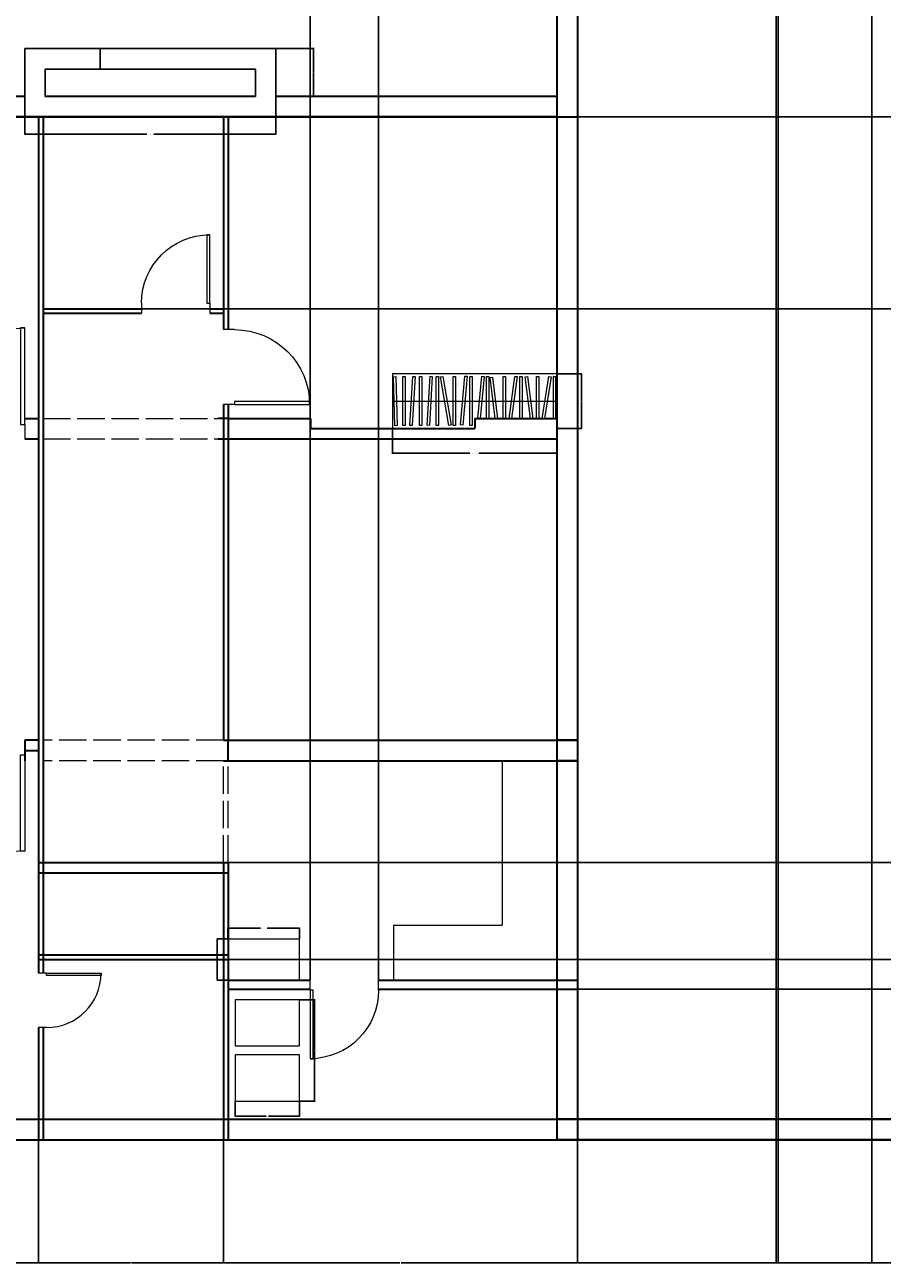
# Model space of a CAD drawing. Units: inches. Extents: x 531915 to 533151, y 849859 to 851471.
# Tile 3 of 7: x 532210 to 532585, y 850315 to 850858. Entities that reach past the tile are written whole.
import ezdxf

# ---------------------------------------------------------------- set-up
doc = ezdxf.new("R2010")
doc.units = ezdxf.units.IN
doc.linetypes.add('ACAD_ISO02W100', pattern=[15, 12, -3])
for name, color, linetype, lineweight in [('A-ANNO-DIMS', 2, 'Continuous', 18), ('A-DOOR', 3, 'Continuous', 18), ('A-FLOR-CASE', 9, 'Continuous', 18), ('A-FLOR-FIXT', 8, 'Continuous', 18), ('A-FLOR-SLAB', 7, 'Continuous', 25), ('A-FURN', 8, 'Continuous', 13), ('A-WALL', 7, 'Continuous', 35), ('A-WALL-OVHD', 7, 'ACAD_ISO02W100', 18)]:
    doc.layers.add(name, color=color, linetype=linetype, lineweight=lineweight)
doc.styles.get("Standard").update_dxf_attribs({"font": 'arial.ttf'})
doc.dimstyles.get("Standard").update_dxf_attribs({"dimtxt": 0.18, "dimasz": 0.18, "dimexe": 0.18, "dimexo": 0.0625, "dimgap": 0.09, "dimtad": 0, "dimtih": 1, "dimtoh": 1, "dimdec": 4, "dimzin": 0, "dimdsep": 46, "dimtxsty": 'Standard', "dimcen": 0.09, "dimadec": 0, "dimazin": 0, "dimtfac": 1, "dimtdec": 4, "dimtofl": 0, "dimtmove": 0, "dimatfit": 3, "dimfxl": 1, "dimtolj": 1, "dimtzin": 0, "dimarcsym": 0})

# ---------------------------------------------------------------- blocks, each defined once
blk = doc.blocks.new('*U2')
for p, q in [((0, 0), (0, -6)), ((40, 0), (40, -6))]:
    blk.add_line(p, q)
blk.add_lwpolyline([(0, 0), (0, 40), (1.75, 40), (1.75, 0)], close=True)
blk.add_arc((0, 0), 40, 0, 90)
blk = doc.blocks.new('WARDROBE-72-RECESSED')
blk.add_line((0, 12), (72, 12))
for points in [[(72, 0), (72, 24), (0, 24), (0, 0), (36.16, 0)], [(37.42, 4.5), (39.13, 22.96), (40.14, 22.87), (38.44, 4.5)], [(41.19, 4.5), (41.19, 22.85), (42.2, 22.85), (42.2, 4.5)], [(45.01, 4.5), (42.84, 22.45), (43.84, 22.58), (46.03, 4.5)], [(48.51, 4.5), (48.51, 22.85), (49.52, 22.85), (49.52, 4.5)], [(51.17, 4.5), (53.59, 22.89), (54.59, 22.76), (52.19, 4.5)], [(55.83, 4.5), (55.83, 22.85), (56.84, 22.85), (56.84, 4.5)], [(60.46, 4.5), (58.13, 22.7), (59.13, 22.83), (61.48, 4.5)], [(63.15, 4.5), (63.15, 22.85), (64.16, 22.85), (64.16, 4.5)], [(65.55, 4.5), (68.56, 22.79), (69.55, 22.63), (66.57, 4.5)], [(70.47, 4.5), (70.47, 22.85), (71.48, 22.85), (71.48, 4.5)]]:
    blk.add_lwpolyline(points)
for points in [[(0.42, 22.75), (1.43, 22.78), (2.11, 1.3), (1.1, 1.27)], [(4.59, 22.85), (5.6, 22.85), (5.6, 1.36), (4.59, 1.36)], [(8.97, 22.89), (9.98, 22.83), (8.71, 1.38), (7.7, 1.44)], [(11.91, 22.85), (12.92, 22.85), (12.92, 1.36), (11.91, 1.36)], [(16.46, 22.95), (17.47, 22.89), (16.21, 1.44), (15.2, 1.5)], [(19.23, 22.85), (20.24, 22.85), (20.24, 1.36), (19.23, 1.36)], [(21.1, 22.62), (22.1, 22.79), (25.68, 1.6), (24.68, 1.43)], [(26.55, 22.85), (27.56, 22.85), (27.56, 1.36), (26.55, 1.36)], [(31.76, 23.02), (32.76, 22.93), (30.78, 1.53), (29.78, 1.63)], [(33.87, 22.85), (34.88, 22.85), (34.88, 1.36), (33.87, 1.36)]]:
    blk.add_lwpolyline(points, close=True)
blk = doc.blocks.new('UTILITY-FIXTURES-PAIR')
for points in [[(0, 24.11), (28.12, 24.11), (28.12, 44.31), (0, 44.31)], [(0, 0), (28.12, 0), (28.12, 20.2), (0, 20.2)]]:
    blk.add_lwpolyline(points, close=True)
blk = doc.blocks.new('SERVICE-LEDGE-110')
for p, q in [((21, 21), (0, 21)), ((0, 21), (0, 0)), ((21, 21), (101, 21)), ((33, 12), (33, 21)), ((101, 21), (110, 21)), ((110, 21), (110, 0)), ((9, 0), (9, 12)), ((9, 12), (21, 12)), ((9, 12), (33, 12)), ((21, 12), (101, 12)), ((101, 0), (101, 12))]:
    blk.add_line(p, q)
blk = doc.blocks.new('COUNTER-L-RETURN')
for p, q in [((47.51, 96), (47.51, 24)), ((0, 24), (47.51, 24)), ((0, 24), (0, 0))]:
    blk.add_line(p, q)
blk = doc.blocks.new('COUNTER-END-RETURN')
for p in [(0, 18), (31.29, 0)]:
    blk.add_line(p, (31.29, 18))
blk = doc.blocks.new('*D17')
at = {"layer": 'A-ANNO-DIMS', "color": 0, "lineweight": -2, "transparency": 16777216}
for p, q in [((532370.8, 850680.81), (532370.8, 850669.89)), ((532442.8, 850680.81), (532442.8, 850669.89)), ((532370.98, 850670.07), (532404.78, 850670.07)), ((532442.62, 850670.07), (532408.83, 850670.07))]:
    blk.add_line(p, q, dxfattribs=at)
at = {"layer": 'A-ANNO-DIMS', "color": 0, "transparency": 16777216}
for points in [[(532370.98, 850670.1), (532370.98, 850670.04), (532370.8, 850670.07)], [(532442.62, 850670.1), (532442.62, 850670.04), (532442.8, 850670.07)]]:
    blk.add_solid(points, dxfattribs=at)
at = {"layer": 'Defpoints', "color": 0, "transparency": 16777216}
for p in [(532370.8, 850680.87), (532442.8, 850680.87), (532442.8, 850670.07)]:
    blk.add_point(p, dxfattribs=at)
at = {"layer": 'A-ANNO-DIMS', "color": 0, "transparency": 16777216, "insert": (532406.8, 850670.07), "char_height": 0.18, "attachment_point": 5}
blk.add_mtext('\\A1;RECESSED WARDROBE 72 TYP.', dxfattribs=at)
blk = doc.blocks.new('*D18')
at = {"layer": 'A-ANNO-DIMS', "color": 0, "lineweight": -2, "transparency": 16777216}
for p, q in [((532442.87, 850704.87), (532453.78, 850704.87)), ((532453.6, 850704.69), (532453.6, 850693.05)), ((532453.6, 850681.05), (532453.6, 850692.69)), ((532442.87, 850680.87), (532453.78, 850680.87))]:
    blk.add_line(p, q, dxfattribs=at)
at = {"layer": 'A-ANNO-DIMS', "color": 0, "transparency": 16777216}
for points in [[(532453.57, 850704.69), (532453.63, 850704.69), (532453.6, 850704.87)], [(532453.57, 850681.05), (532453.63, 850681.05), (532453.6, 850680.87)]]:
    blk.add_solid(points, dxfattribs=at)
at = {"layer": 'Defpoints', "color": 0, "transparency": 16777216}
for p in [(532442.8, 850704.87), (532453.6, 850704.87), (532442.8, 850680.87)]:
    blk.add_point(p, dxfattribs=at)
at = {"layer": 'A-ANNO-DIMS', "color": 0, "transparency": 16777216, "insert": (532453.6, 850692.87), "char_height": 0.18, "attachment_point": 5}
blk.add_mtext('\\A1;24 TYP.', dxfattribs=at)
blk = doc.blocks.new('*D23')
at = {"layer": 'A-ANNO-DIMS', "color": 0, "lineweight": -2, "transparency": 16777216}
for p, q in [((532330.16, 850430.7), (532336.93, 850430.7)), ((532336.75, 850430.52), (532336.75, 850408.72)), ((532336.75, 850386.57), (532336.75, 850408.36)), ((532330.16, 850386.39), (532336.93, 850386.39))]:
    blk.add_line(p, q, dxfattribs=at)
at = {"layer": 'A-ANNO-DIMS', "color": 0, "transparency": 16777216}
for points in [[(532336.72, 850430.52), (532336.78, 850430.52), (532336.75, 850430.7)], [(532336.72, 850386.57), (532336.78, 850386.57), (532336.75, 850386.39)]]:
    blk.add_solid(points, dxfattribs=at)
at = {"layer": 'Defpoints', "color": 0, "transparency": 16777216}
for p in [(532330.1, 850430.7), (532336.75, 850430.7), (532330.1, 850386.39)]:
    blk.add_point(p, dxfattribs=at)
at = {"layer": 'A-ANNO-DIMS', "color": 0, "transparency": 16777216, "insert": (532336.75, 850408.54), "char_height": 0.18, "attachment_point": 5}
blk.add_mtext('\\A1;UTILITY FIXTURES 44 TYP.', dxfattribs=at)
blk = doc.blocks.new('*D24')
at = {"layer": 'A-ANNO-DIMS', "color": 0, "lineweight": -2, "transparency": 16777216}
for p, q in [((532301.98, 850386.32), (532301.98, 850379.56)), ((532330.1, 850386.32), (532330.1, 850379.56)), ((532302.16, 850379.74), (532315.51, 850379.74)), ((532329.92, 850379.74), (532316.57, 850379.74))]:
    blk.add_line(p, q, dxfattribs=at)
at = {"layer": 'A-ANNO-DIMS', "color": 0, "transparency": 16777216}
for points in [[(532302.16, 850379.77), (532302.16, 850379.71), (532301.98, 850379.74)], [(532329.92, 850379.77), (532329.92, 850379.71), (532330.1, 850379.74)]]:
    blk.add_solid(points, dxfattribs=at)
at = {"layer": 'Defpoints', "color": 0, "transparency": 16777216}
for p in [(532301.98, 850386.39), (532330.1, 850386.39), (532330.1, 850379.74)]:
    blk.add_point(p, dxfattribs=at)
at = {"layer": 'A-ANNO-DIMS', "color": 0, "transparency": 16777216, "insert": (532316.04, 850379.74), "char_height": 0.18, "attachment_point": 5}
blk.add_mtext('\\A1;28 TYP.', dxfattribs=at)
blk = doc.blocks.new('*D27')
at = {"layer": 'A-ANNO-DIMS', "color": 0, "lineweight": -2, "transparency": 16777216}
for p, q in [((532298.8, 850457.44), (532298.8, 850462.25)), ((532298.98, 850462.07), (532312.97, 850462.07)), ((532329.92, 850462.07), (532315.94, 850462.07)), ((532330.1, 850457.44), (532330.1, 850462.25))]:
    blk.add_line(p, q, dxfattribs=at)
at = {"layer": 'A-ANNO-DIMS', "color": 0, "transparency": 16777216}
for points in [[(532298.98, 850462.1), (532298.98, 850462.04), (532298.8, 850462.07)], [(532329.92, 850462.1), (532329.92, 850462.04), (532330.1, 850462.07)]]:
    blk.add_solid(points, dxfattribs=at)
at = {"layer": 'Defpoints', "color": 0, "transparency": 16777216}
for p in [(532330.1, 850462.07), (532298.8, 850457.37), (532330.1, 850457.37)]:
    blk.add_point(p, dxfattribs=at)
at = {"layer": 'A-ANNO-DIMS', "color": 0, "transparency": 16777216, "insert": (532314.45, 850462.07), "char_height": 0.18, "attachment_point": 5}
blk.add_mtext('\\A1;COUNTER END 31 TYP.', dxfattribs=at)
blk = doc.blocks.new('*D28')
at = {"layer": 'A-ANNO-DIMS', "color": 0, "lineweight": -2, "transparency": 16777216}
for p, q in [((532298.74, 850457.37), (532293.93, 850457.37)), ((532294.11, 850457.19), (532294.11, 850448.56)), ((532294.11, 850439.55), (532294.11, 850448.19)), ((532298.74, 850439.37), (532293.93, 850439.37))]:
    blk.add_line(p, q, dxfattribs=at)
at = {"layer": 'A-ANNO-DIMS', "color": 0, "transparency": 16777216}
for points in [[(532294.08, 850457.19), (532294.14, 850457.19), (532294.11, 850457.37)], [(532294.08, 850439.55), (532294.14, 850439.55), (532294.11, 850439.37)]]:
    blk.add_solid(points, dxfattribs=at)
at = {"layer": 'Defpoints', "color": 0, "transparency": 16777216}
for p in [(532294.11, 850457.37), (532298.8, 850457.37), (532298.8, 850439.37)]:
    blk.add_point(p, dxfattribs=at)
at = {"layer": 'A-ANNO-DIMS', "color": 0, "transparency": 16777216, "insert": (532294.11, 850448.37), "char_height": 0.18, "attachment_point": 5}
blk.add_mtext('\\A1;18 TYP.', dxfattribs=at)
blk = doc.blocks.new('*D35')
at = {"layer": 'A-ANNO-DIMS', "color": 0, "lineweight": -2, "transparency": 16777216}
for p, q in [((532209.8, 850826.31), (532209.8, 850809.69)), ((532319.8, 850826.31), (532319.8, 850809.69)), ((532209.98, 850809.87), (532263.26, 850809.87)), ((532319.62, 850809.87), (532266.35, 850809.87))]:
    blk.add_line(p, q, dxfattribs=at)
at = {"layer": 'A-ANNO-DIMS', "color": 0, "transparency": 16777216}
for points in [[(532209.98, 850809.9), (532209.98, 850809.84), (532209.8, 850809.87)], [(532319.62, 850809.9), (532319.62, 850809.84), (532319.8, 850809.87)]]:
    blk.add_solid(points, dxfattribs=at)
at = {"layer": 'Defpoints', "color": 0, "transparency": 16777216}
for p in [(532209.8, 850826.37), (532319.8, 850826.37), (532319.8, 850809.87)]:
    blk.add_point(p, dxfattribs=at)
at = {"layer": 'A-ANNO-DIMS', "color": 0, "transparency": 16777216, "insert": (532264.8, 850809.87), "char_height": 0.18, "attachment_point": 5}
blk.add_mtext('\\A1;SERVICE SLAB 110 TYP.', dxfattribs=at)
blk = doc.blocks.new('*D36')
at = {"layer": 'A-ANNO-DIMS', "color": 0, "lineweight": -2, "transparency": 16777216}
for p, q in [((532319.87, 850847.37), (532336.48, 850847.37)), ((532336.3, 850847.19), (532336.3, 850837.05)), ((532336.3, 850826.55), (532336.3, 850836.69)), ((532319.87, 850826.37), (532336.48, 850826.37))]:
    blk.add_line(p, q, dxfattribs=at)
at = {"layer": 'A-ANNO-DIMS', "color": 0, "transparency": 16777216}
for points in [[(532336.27, 850847.19), (532336.33, 850847.19), (532336.3, 850847.37)], [(532336.27, 850826.55), (532336.33, 850826.55), (532336.3, 850826.37)]]:
    blk.add_solid(points, dxfattribs=at)
at = {"layer": 'Defpoints', "color": 0, "transparency": 16777216}
for p in [(532319.8, 850847.37), (532336.3, 850847.37), (532319.8, 850826.37)]:
    blk.add_point(p, dxfattribs=at)
at = {"layer": 'A-ANNO-DIMS', "color": 0, "transparency": 16777216, "insert": (532336.3, 850836.87), "char_height": 0.18, "attachment_point": 5}
blk.add_mtext('\\A1;21 TYP.', dxfattribs=at)
blk = doc.blocks.new('*D41')
at = {"layer": 'A-ANNO-DIMS', "color": 0, "lineweight": -2, "transparency": 16777216}
for p, q in [((532451.74, 850922.23), (531968.71, 850922.23)), ((531968.89, 850922.05), (531968.89, 850874.49)), ((531968.89, 850826.55), (531968.89, 850874.12)), ((532062.74, 850826.37), (531968.71, 850826.37))]:
    blk.add_line(p, q, dxfattribs=at)
at = {"layer": 'A-ANNO-DIMS', "color": 0, "transparency": 16777216}
for points in [[(531968.86, 850922.05), (531968.92, 850922.05), (531968.89, 850922.23)], [(531968.86, 850826.55), (531968.92, 850826.55), (531968.89, 850826.37)]]:
    blk.add_solid(points, dxfattribs=at)
at = {"layer": 'Defpoints', "color": 0, "transparency": 16777216}
for p in [(532451.8, 850922.23), (531968.89, 850826.37), (532062.8, 850826.37)]:
    blk.add_point(p, dxfattribs=at)
at = {"layer": 'A-ANNO-DIMS', "color": 0, "transparency": 16777216, "insert": (531968.89, 850874.3), "char_height": 0.18, "attachment_point": 5}
blk.add_mtext('\\A1;95.86', dxfattribs=at)
blk = doc.blocks.new('*D42')
at = {"layer": 'A-ANNO-DIMS', "color": 0, "lineweight": -2, "transparency": 16777216}
for p, q in [((532451.8, 850369.31), (532451.8, 850315.34)), ((532667.8, 850369.31), (532667.8, 850315.34)), ((532451.98, 850315.52), (532559.51, 850315.52)), ((532667.62, 850315.52), (532560.1, 850315.52))]:
    blk.add_line(p, q, dxfattribs=at)
at = {"layer": 'A-ANNO-DIMS', "color": 0, "transparency": 16777216}
for points in [[(532451.98, 850315.55), (532451.98, 850315.49), (532451.8, 850315.52)], [(532667.62, 850315.55), (532667.62, 850315.49), (532667.8, 850315.52)]]:
    blk.add_solid(points, dxfattribs=at)
at = {"layer": 'Defpoints', "color": 0, "transparency": 16777216}
for p in [(532451.8, 850369.37), (532667.8, 850369.37), (532667.8, 850315.52)]:
    blk.add_point(p, dxfattribs=at)
at = {"layer": 'A-ANNO-DIMS', "color": 0, "transparency": 16777216, "insert": (532559.8, 850315.52), "char_height": 0.18, "attachment_point": 5}
blk.add_mtext('\\A1;216', dxfattribs=at)
blk = doc.blocks.new('*D60')
at = {"layer": 'A-ANNO-DIMS', "color": 0, "lineweight": -2, "transparency": 16777216}
for p, q in [((532062.8, 850369.31), (532062.8, 850315.34)), ((532215.8, 850369.31), (532215.8, 850315.34)), ((532062.98, 850315.52), (532139.02, 850315.52)), ((532215.62, 850315.52), (532139.59, 850315.52))]:
    blk.add_line(p, q, dxfattribs=at)
at = {"layer": 'A-ANNO-DIMS', "color": 0, "transparency": 16777216}
for points in [[(532062.98, 850315.55), (532062.98, 850315.49), (532062.8, 850315.52)], [(532215.62, 850315.55), (532215.62, 850315.49), (532215.8, 850315.52)]]:
    blk.add_solid(points, dxfattribs=at)
at = {"layer": 'Defpoints', "color": 0, "transparency": 16777216}
for p in [(532062.8, 850369.37), (532215.8, 850369.37), (532215.8, 850315.52)]:
    blk.add_point(p, dxfattribs=at)
at = {"layer": 'A-ANNO-DIMS', "color": 0, "transparency": 16777216, "insert": (532139.3, 850315.52), "char_height": 0.18, "attachment_point": 5}
blk.add_mtext('\\A1;153', dxfattribs=at)
blk = doc.blocks.new('*D61')
at = {"layer": 'A-ANNO-DIMS', "color": 0, "lineweight": -2, "transparency": 16777216}
for p, q in [((532215.8, 850369.31), (532215.8, 850315.34)), ((532296.8, 850369.31), (532296.8, 850315.34)), ((532215.98, 850315.52), (532256.1, 850315.52)), ((532296.62, 850315.52), (532256.51, 850315.52))]:
    blk.add_line(p, q, dxfattribs=at)
at = {"layer": 'A-ANNO-DIMS', "color": 0, "transparency": 16777216}
for points in [[(532215.98, 850315.55), (532215.98, 850315.49), (532215.8, 850315.52)], [(532296.62, 850315.55), (532296.62, 850315.49), (532296.8, 850315.52)]]:
    blk.add_solid(points, dxfattribs=at)
at = {"layer": 'Defpoints', "color": 0, "transparency": 16777216}
for p in [(532215.8, 850369.37), (532296.8, 850369.37), (532296.8, 850315.52)]:
    blk.add_point(p, dxfattribs=at)
at = {"layer": 'A-ANNO-DIMS', "color": 0, "transparency": 16777216, "insert": (532256.3, 850315.52), "char_height": 0.18, "attachment_point": 5}
blk.add_mtext('\\A1;81', dxfattribs=at)
blk = doc.blocks.new('*D62')
at = {"layer": 'A-ANNO-DIMS', "color": 0, "lineweight": -2, "transparency": 16777216}
for p, q in [((532296.8, 850369.31), (532296.8, 850315.34)), ((532451.8, 850369.31), (532451.8, 850315.34)), ((532296.98, 850315.52), (532374.02, 850315.52)), ((532451.62, 850315.52), (532374.59, 850315.52))]:
    blk.add_line(p, q, dxfattribs=at)
at = {"layer": 'A-ANNO-DIMS', "color": 0, "transparency": 16777216}
for points in [[(532296.98, 850315.55), (532296.98, 850315.49), (532296.8, 850315.52)], [(532451.62, 850315.55), (532451.62, 850315.49), (532451.8, 850315.52)]]:
    blk.add_solid(points, dxfattribs=at)
at = {"layer": 'Defpoints', "color": 0, "transparency": 16777216}
for p in [(532296.8, 850369.37), (532451.8, 850369.37), (532451.8, 850315.52)]:
    blk.add_point(p, dxfattribs=at)
at = {"layer": 'A-ANNO-DIMS', "color": 0, "transparency": 16777216, "insert": (532374.3, 850315.52), "char_height": 0.18, "attachment_point": 5}
blk.add_mtext('\\A1;155', dxfattribs=at)
blk = doc.blocks.new('*D67')
at = {"layer": 'A-ANNO-DIMS', "color": 0, "lineweight": -2, "transparency": 16777216}
for p, q in [((532451.87, 850435.37), (533150.9, 850435.37)), ((533150.72, 850435.19), (533150.72, 850407.06)), ((533150.72, 850378.55), (533150.72, 850406.69)), ((532442.87, 850378.37), (533150.9, 850378.37))]:
    blk.add_line(p, q, dxfattribs=at)
at = {"layer": 'A-ANNO-DIMS', "color": 0, "transparency": 16777216}
for points in [[(533150.69, 850435.19), (533150.75, 850435.19), (533150.72, 850435.37)], [(533150.69, 850378.55), (533150.75, 850378.55), (533150.72, 850378.37)]]:
    blk.add_solid(points, dxfattribs=at)
at = {"layer": 'Defpoints', "color": 0, "transparency": 16777216}
for p in [(532451.8, 850435.37), (532442.8, 850378.37), (533150.72, 850378.37)]:
    blk.add_point(p, dxfattribs=at)
at = {"layer": 'A-ANNO-DIMS', "color": 0, "transparency": 16777216, "insert": (533150.72, 850406.87), "char_height": 0.18, "attachment_point": 5}
blk.add_mtext('\\A1;57', dxfattribs=at)
blk = doc.blocks.new('*D72')
at = {"layer": 'A-ANNO-DIMS', "color": 0, "lineweight": -2, "transparency": 16777216}
for p, q in [((532451.8, 850931.17), (532451.8, 850315.34)), ((532539.8, 850931.17), (532539.8, 850315.34)), ((532451.98, 850315.52), (532495.59, 850315.52)), ((532539.62, 850315.52), (532496.02, 850315.52))]:
    blk.add_line(p, q, dxfattribs=at)
at = {"layer": 'A-ANNO-DIMS', "color": 0, "transparency": 16777216}
for points in [[(532451.98, 850315.55), (532451.98, 850315.49), (532451.8, 850315.52)], [(532539.62, 850315.55), (532539.62, 850315.49), (532539.8, 850315.52)]]:
    blk.add_solid(points, dxfattribs=at)
at = {"layer": 'Defpoints', "color": 0, "transparency": 16777216}
for p in [(532451.8, 850931.23), (532539.8, 850931.23), (532539.8, 850315.52)]:
    blk.add_point(p, dxfattribs=at)
at = {"layer": 'A-ANNO-DIMS', "color": 0, "transparency": 16777216, "insert": (532495.8, 850315.52), "char_height": 0.18, "attachment_point": 5}
blk.add_mtext('\\A1;88', dxfattribs=at)
blk = doc.blocks.new('*D73')
at = {"layer": 'A-ANNO-DIMS', "color": 0, "lineweight": -2, "transparency": 16777216}
for p, q in [((532539.8, 850931.17), (532539.8, 850315.34)), ((532580.8, 850931.17), (532580.8, 850315.34)), ((532539.98, 850315.52), (532560.1, 850315.52)), ((532580.62, 850315.52), (532560.51, 850315.52))]:
    blk.add_line(p, q, dxfattribs=at)
at = {"layer": 'A-ANNO-DIMS', "color": 0, "transparency": 16777216}
for points in [[(532539.98, 850315.55), (532539.98, 850315.49), (532539.8, 850315.52)], [(532580.62, 850315.55), (532580.62, 850315.49), (532580.8, 850315.52)]]:
    blk.add_solid(points, dxfattribs=at)
at = {"layer": 'Defpoints', "color": 0, "transparency": 16777216}
for p in [(532539.8, 850931.23), (532580.8, 850931.23), (532580.8, 850315.52)]:
    blk.add_point(p, dxfattribs=at)
at = {"layer": 'A-ANNO-DIMS', "color": 0, "transparency": 16777216, "insert": (532560.3, 850315.52), "char_height": 0.18, "attachment_point": 5}
blk.add_mtext('\\A1;41', dxfattribs=at)
blk = doc.blocks.new('*D77')
at = {"layer": 'A-ANNO-DIMS', "color": 0, "lineweight": -2, "transparency": 16777216}
for p, q in [((532215.87, 850817.37), (533150.9, 850817.37)), ((533150.72, 850817.19), (533150.72, 850775.56)), ((533150.72, 850733.55), (533150.72, 850775.19)), ((532217.87, 850733.37), (533150.9, 850733.37))]:
    blk.add_line(p, q, dxfattribs=at)
at = {"layer": 'A-ANNO-DIMS', "color": 0, "transparency": 16777216}
for points in [[(533150.69, 850817.19), (533150.75, 850817.19), (533150.72, 850817.37)], [(533150.69, 850733.55), (533150.75, 850733.55), (533150.72, 850733.37)]]:
    blk.add_solid(points, dxfattribs=at)
at = {"layer": 'Defpoints', "color": 0, "transparency": 16777216}
for p in [(532215.8, 850817.37), (532217.8, 850733.37), (533150.72, 850733.37)]:
    blk.add_point(p, dxfattribs=at)
at = {"layer": 'A-ANNO-DIMS', "color": 0, "transparency": 16777216, "insert": (533150.72, 850775.37), "char_height": 0.18, "attachment_point": 5}
blk.add_mtext('\\A1;84', dxfattribs=at)
blk = doc.blocks.new('*D78')
at = {"layer": 'A-ANNO-DIMS', "color": 0, "lineweight": -2, "transparency": 16777216}
for p, q in [((532451.8, 851196.17), (532451.8, 850315.34)), ((532538.8, 851196.17), (532538.8, 850315.34)), ((532451.98, 850315.52), (532495.09, 850315.52)), ((532538.62, 850315.52), (532495.52, 850315.52))]:
    blk.add_line(p, q, dxfattribs=at)
at = {"layer": 'A-ANNO-DIMS', "color": 0, "transparency": 16777216}
for points in [[(532451.98, 850315.55), (532451.98, 850315.49), (532451.8, 850315.52)], [(532538.62, 850315.55), (532538.62, 850315.49), (532538.8, 850315.52)]]:
    blk.add_solid(points, dxfattribs=at)
at = {"layer": 'Defpoints', "color": 0, "transparency": 16777216}
for p in [(532451.8, 851196.23), (532538.8, 851196.23), (532538.8, 850315.52)]:
    blk.add_point(p, dxfattribs=at)
at = {"layer": 'A-ANNO-DIMS', "color": 0, "transparency": 16777216, "insert": (532495.3, 850315.52), "char_height": 0.18, "attachment_point": 5}
blk.add_mtext('\\A1;87', dxfattribs=at)
blk = doc.blocks.new('*D84')
at = {"layer": 'A-ANNO-DIMS', "color": 0, "lineweight": -2, "transparency": 16777216}
for p, q in [((532215.87, 850490.87), (533150.9, 850490.87)), ((533150.72, 850490.69), (533150.72, 850469.81)), ((533150.72, 850448.55), (533150.72, 850469.44)), ((532215.87, 850448.37), (533150.9, 850448.37))]:
    blk.add_line(p, q, dxfattribs=at)
at = {"layer": 'A-ANNO-DIMS', "color": 0, "transparency": 16777216}
for points in [[(533150.69, 850490.69), (533150.75, 850490.69), (533150.72, 850490.87)], [(533150.69, 850448.55), (533150.75, 850448.55), (533150.72, 850448.37)]]:
    blk.add_solid(points, dxfattribs=at)
at = {"layer": 'Defpoints', "color": 0, "transparency": 16777216}
for p in [(532215.8, 850490.87), (532215.8, 850448.37), (533150.72, 850448.37)]:
    blk.add_point(p, dxfattribs=at)
at = {"layer": 'A-ANNO-DIMS', "color": 0, "transparency": 16777216, "insert": (533150.72, 850469.62), "char_height": 0.18, "attachment_point": 5}
blk.add_mtext('\\A1;42.5', dxfattribs=at)
blk = doc.blocks.new('*D85')
at = {"layer": 'A-ANNO-DIMS', "color": 0, "lineweight": -2, "transparency": 16777216}
for p, q in [((532334.8, 850439.44), (532334.8, 851470.96)), ((532334.98, 851470.78), (532349.32, 851470.78)), ((532364.58, 851470.78), (532350.25, 851470.78)), ((532364.76, 850439.44), (532364.76, 851470.96))]:
    blk.add_line(p, q, dxfattribs=at)
at = {"layer": 'A-ANNO-DIMS', "color": 0, "transparency": 16777216}
for points in [[(532334.98, 851470.81), (532334.98, 851470.75), (532334.8, 851470.78)], [(532364.58, 851470.81), (532364.58, 851470.75), (532364.76, 851470.78)]]:
    blk.add_solid(points, dxfattribs=at)
at = {"layer": 'Defpoints', "color": 0, "transparency": 16777216}
for p in [(532364.76, 851470.78), (532334.8, 850439.37), (532364.76, 850439.37)]:
    blk.add_point(p, dxfattribs=at)
at = {"layer": 'A-ANNO-DIMS', "color": 0, "transparency": 16777216, "insert": (532349.78, 851470.78), "char_height": 0.18, "attachment_point": 5}
blk.add_mtext('\\A1;29.954', dxfattribs=at)

msp = doc.modelspace()

# ---------------------------------------------------------------- linework, layer by layer
at = {"layer": 'A-WALL'}
for p, q in [((532442.8048, 850946.374), (532442.8048, 850826.374)), ((532442.8048, 850931.2344), (532442.8048, 850369.374)), ((532451.8048, 850931.2344), (532451.8048, 850369.374)), ((532209.8048, 850826.374), (532062.8048, 850826.374)), ((532310.8048, 850826.374), (532218.8048, 850826.374)), ((532442.8048, 850826.374), (532319.8048, 850826.374)), ((532442.8048, 850817.374), (532062.8048, 850817.374)), ((532062.8048, 850817.374), (532451.8048, 850817.374)), ((532215.8048, 850817.374), (532215.8048, 850442.374)), ((532217.8048, 850817.374), (532217.8048, 850442.374)), ((532217.8048, 850817.374), (532296.8048, 850817.374)), ((532296.8048, 850817.374), (532296.8048, 850724.227)), ((532298.8048, 850817.374), (532298.8048, 850724.227)), ((532217.8048, 850733.374), (532260.9212, 850733.374)), ((532217.8048, 850731.374), (532260.9212, 850731.374)), ((532290.8048, 850733.374), (532296.8048, 850733.374)), ((532290.8048, 850731.374), (532296.8048, 850731.374)), ((532296.8048, 850691.374), (532296.8048, 850544.374)), ((532298.8048, 850691.374), (532298.8048, 850544.374)), ((532209.8048, 850685.374), (532215.8048, 850685.374)), ((532299.125, 850685.374), (532294.3048, 850685.374)), ((532299.125, 850685.374), (532334.9649, 850685.374)), ((532299.125, 850685.374), (532334.9649, 850685.374)), ((532299.125, 850685.374), (532334.9649, 850685.374)), ((532334.9649, 850685.374), (532334.9649, 850680.874)), ((532334.9649, 850680.874), (532406.9649, 850680.874)), ((532406.9649, 850685.374), (532442.8048, 850685.374)), ((532406.9649, 850685.374), (532406.9649, 850680.874)), ((532209.8048, 850676.374), (532215.8048, 850676.374)), ((532294.3048, 850676.374), (532442.8048, 850676.374)), ((532298.8048, 850676.374), (532442.8048, 850676.374)), ((532209.8048, 850544.374), (532209.8048, 850535.374)), ((532215.8048, 850544.374), (532209.8048, 850544.374)), ((532209.8048, 850539.874), (532215.8048, 850539.874)), ((532215.8048, 850544.374), (532215.8048, 850535.374)), ((532296.8048, 850544.374), (532451.8048, 850544.374)), ((532298.8048, 850535.374), (532298.8048, 850544.374)), ((532451.8048, 850544.374), (532442.8048, 850544.374)), ((532296.8048, 850535.374), (532451.8048, 850535.374)), ((532451.8048, 850535.374), (532442.8048, 850535.374)), ((532215.8048, 850490.874), (532298.8048, 850490.874)), ((532296.8048, 850490.874), (532296.8048, 850369.374)), ((532298.8048, 850490.874), (532298.8048, 850369.374)), ((532215.8048, 850486.374), (532298.8048, 850486.374)), ((532215.8048, 850450.374), (532298.8048, 850450.374)), ((532215.8048, 850448.374), (532298.8048, 850448.374)), ((532298.8048, 850439.374), (532334.8048, 850439.374)), ((532364.7592, 850439.374), (532451.8048, 850439.374)), ((532298.8048, 850435.374), (532334.8048, 850435.374)), ((532364.7592, 850435.374), (532451.8048, 850435.374)), ((532215.8048, 850418.5523), (532215.8048, 850369.374)), ((532217.8048, 850418.5523), (532217.8048, 850369.374)), ((532062.8048, 850378.374), (532676.8048, 850378.374)), ((533056.8048, 850378.374), (532442.8048, 850378.374)), ((532062.8048, 850369.374), (532676.8048, 850369.374)), ((533056.8048, 850369.374), (532442.8048, 850369.374))]:
    msp.add_line(p, q, dxfattribs=at)
at = {"layer": 'A-WALL-OVHD'}
for p, q in [((532217.8048, 850685.374), (532296.8048, 850685.374)), ((532217.8048, 850676.374), (532296.8048, 850676.374)), ((532296.8048, 850544.374), (532217.8048, 850544.374)), ((532296.8048, 850535.374), (532217.8048, 850535.374)), ((532296.8048, 850490.874), (532296.8048, 850535.374)), ((532298.8048, 850490.874), (532298.8048, 850535.374))]:
    msp.add_line(p, q, dxfattribs=at)

# ---------------------------------------------------------------- block references
at = {"layer": 'A-DOOR'}
for p, xscale, yscale, zscale in [((532290.8048, 850735.8565), -0.7470890379753774, 0.7470890379753774, 0.7470890379753774), ((532209.8048, 850682.7117), -1.056294156906435, 1.056294156906435, 1.056294156906435)]:
    msp.add_blockref('*U2', p, dxfattribs=dict(at, xscale=xscale, yscale=yscale, zscale=zscale))
for p, xscale, yscale, zscale, rotation in [((532301.6967, 850691.374), -0.8213266256042635, 0.8213266256042635, 0.8213266256042635, 270), ((532209.8048, 850538.0362), 1.056294156906435, 1.056294156906435, 1.056294156906435, 180), ((532219.378, 850442.374), 0.5955413682082586, 0.5955413682082586, 0.5955413682082586, 270), ((532334.8048, 850434.8808), -0.7488601199280389, 0.7488601199280389, 0.7488601199280389, 180)]:
    msp.add_blockref('*U2', p, dxfattribs=dict(at, xscale=xscale, yscale=yscale, zscale=zscale, rotation=rotation))
at = {"layer": 'A-FLOR-CASE'}
for name, p in [('COUNTER-L-RETURN', (532371.2933, 850439.374)), ('COUNTER-END-RETURN', (532298.8048, 850439.374))]:
    msp.add_blockref(name, p, dxfattribs=at)
at = {"layer": 'A-FLOR-FIXT'}
msp.add_blockref('UTILITY-FIXTURES-PAIR', (532301.9813, 850386.385), dxfattribs=at)
at = {"layer": 'A-FLOR-SLAB'}
msp.add_blockref('SERVICE-LEDGE-110', (532209.8048, 850826.374), dxfattribs=at)
at = {"layer": 'A-FURN'}
msp.add_blockref('WARDROBE-72-RECESSED', (532370.8048, 850680.874), dxfattribs=at)

# ---------------------------------------------------------------- dimensions: what is measured, and where the dimension line sits
at = {"layer": 'A-ANNO-DIMS'}
for base, p1, p2, override, picture, middle in [((532364.7592, 851470.7848), (532334.8048, 850439.374), (532364.7592, 850439.374), {"dimdec": 3, "dimlfac": 1, "dimrnd": 0, "dimzin": 0, "dimdsep": 46, "dimlunit": 2}, '*D85', (532349.782, 851470.7848)), ((532538.8048, 850315.524), (532451.8048, 851196.2344), (532538.8048, 851196.2344), {"dimdec": 0, "dimlfac": 1, "dimrnd": 0, "dimzin": 0, "dimdsep": 46, "dimlunit": 2}, '*D78', (532495.3048, 850315.524)), ((532539.8048, 850315.524), (532451.8048, 850931.2344), (532539.8048, 850931.2344), {"dimdec": 0, "dimlfac": 1, "dimrnd": 0, "dimzin": 0, "dimdsep": 46, "dimlunit": 2}, '*D72', (532495.8048, 850315.524)), ((532580.8048, 850315.524), (532539.8048, 850931.2344), (532580.8048, 850931.2344), {"dimdec": 0, "dimlfac": 1, "dimrnd": 0, "dimzin": 0, "dimdsep": 46, "dimlunit": 2}, '*D73', (532560.3048, 850315.524)), ((532215.8048, 850315.524), (532062.8048, 850369.374), (532215.8048, 850369.374), {"dimdec": 0, "dimlfac": 1, "dimrnd": 0, "dimzin": 0, "dimdsep": 46, "dimlunit": 2}, '*D60', (532139.3048, 850315.524)), ((532296.8048, 850315.524), (532215.8048, 850369.374), (532296.8048, 850369.374), {"dimdec": 0, "dimlfac": 1, "dimrnd": 0, "dimzin": 0, "dimdsep": 46, "dimlunit": 2}, '*D61', (532256.3048, 850315.524)), ((532451.8048, 850315.524), (532296.8048, 850369.374), (532451.8048, 850369.374), {"dimdec": 0, "dimlfac": 1, "dimrnd": 0, "dimzin": 0, "dimdsep": 46, "dimlunit": 2}, '*D62', (532374.3048, 850315.524)), ((532667.8048, 850315.524), (532451.8048, 850369.374), (532667.8048, 850369.374), {"dimdec": 0, "dimlfac": 1, "dimrnd": 0, "dimzin": 0, "dimdsep": 46, "dimlunit": 2}, '*D42', (532559.8048, 850315.524))]:
    dim = msp.add_linear_dim(base=base, p1=p1, p2=p2, dimstyle='Standard', override=override, dxfattribs=at)
    dim.commit()
    dim.dimension.update_dxf_attribs({"geometry": picture, "text_midpoint": middle})
for base, p1, p2, override, picture, middle in [((531968.8939, 850826.374), (532451.8048, 850922.2344), (532062.8048, 850826.374), {"dimdec": 2, "dimlfac": 1, "dimrnd": 0, "dimzin": 0, "dimdsep": 46, "dimlunit": 2}, '*D41', (531968.8939, 850874.3042)), ((533150.7156, 850733.374), (532215.8048, 850817.374), (532217.8048, 850733.374), {"dimdec": 0, "dimlfac": 1, "dimrnd": 0, "dimzin": 0, "dimdsep": 46, "dimlunit": 2}, '*D77', (533150.7156, 850775.374)), ((533150.7156, 850448.374), (532215.8048, 850490.874), (532215.8048, 850448.374), {"dimdec": 1, "dimlfac": 1, "dimrnd": 0, "dimzin": 0, "dimdsep": 46, "dimlunit": 2}, '*D84', (533150.7156, 850469.624)), ((533150.7156, 850378.374), (532451.8048, 850435.374), (532442.8048, 850378.374), {"dimdec": 0, "dimlfac": 1, "dimrnd": 0, "dimzin": 0, "dimdsep": 46, "dimlunit": 2}, '*D67', (533150.7156, 850406.874))]:
    dim = msp.add_linear_dim(base=base, p1=p1, p2=p2, angle=90, dimstyle='Standard', override=override, dxfattribs=at)
    dim.commit()
    dim.dimension.update_dxf_attribs({"geometry": picture, "text_midpoint": middle})
for base, p1, p2, text, picture, middle in [((532336.3048, 850847.374), (532319.8048, 850826.374), (532319.8048, 850847.374), '<> TYP.', '*D36', (532336.3048, 850836.874)), ((532453.6048, 850704.874), (532442.8048, 850680.874), (532442.8048, 850704.874), '<> TYP.', '*D18', (532453.6048, 850692.874)), ((532294.1107, 850457.374), (532298.8048, 850439.374), (532298.8048, 850457.374), '<> TYP.', '*D28', (532294.1107, 850448.374)), ((532336.7453, 850430.6957), (532330.0987, 850386.385), (532330.0987, 850430.6957), 'UTILITY FIXTURES <> TYP.', '*D23', (532336.7453, 850408.5403))]:
    dim = msp.add_linear_dim(base=base, p1=p1, p2=p2, angle=90, text=text, dimstyle='Standard', override={"dimdec": 0, "dimlfac": 1, "dimrnd": 0, "dimzin": 0, "dimdsep": 46, "dimlunit": 2}, dxfattribs=at)
    dim.commit()
    dim.dimension.update_dxf_attribs({"geometry": picture, "text_midpoint": middle})
for base, p1, p2, text, picture, middle in [((532319.8048, 850809.874), (532209.8048, 850826.374), (532319.8048, 850826.374), 'SERVICE SLAB <> TYP.', '*D35', (532264.8048, 850809.874)), ((532442.8048, 850670.074), (532370.8048, 850680.874), (532442.8048, 850680.874), 'RECESSED WARDROBE <> TYP.', '*D17', (532406.8048, 850670.074)), ((532330.0987, 850462.0681), (532298.8048, 850457.374), (532330.0987, 850457.374), 'COUNTER END <> TYP.', '*D27', (532314.4518, 850462.0681)), ((532330.0987, 850379.7384), (532301.9813, 850386.385), (532330.0987, 850386.385), '<> TYP.', '*D24', (532316.04, 850379.7384))]:
    dim = msp.add_linear_dim(base=base, p1=p1, p2=p2, text=text, dimstyle='Standard', override={"dimdec": 0, "dimlfac": 1, "dimrnd": 0, "dimzin": 0, "dimdsep": 46, "dimlunit": 2}, dxfattribs=at)
    dim.commit()
    dim.dimension.update_dxf_attribs({"geometry": picture, "text_midpoint": middle})

doc.saveas('drawing.dxf')
